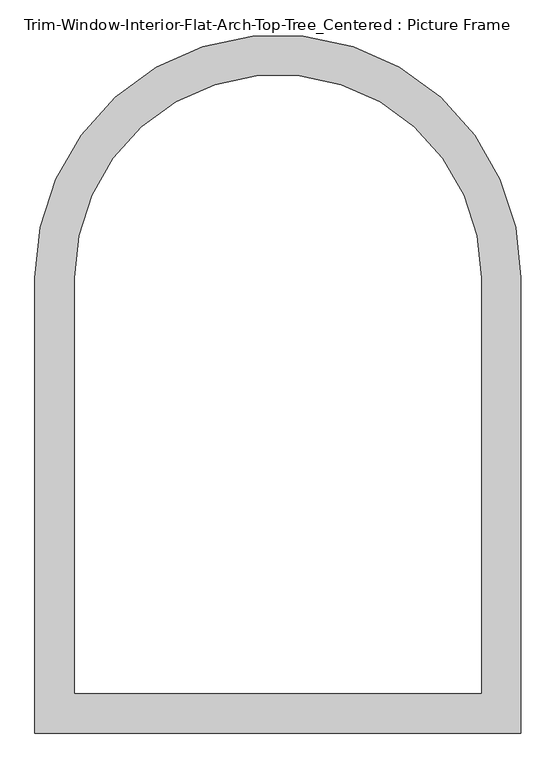
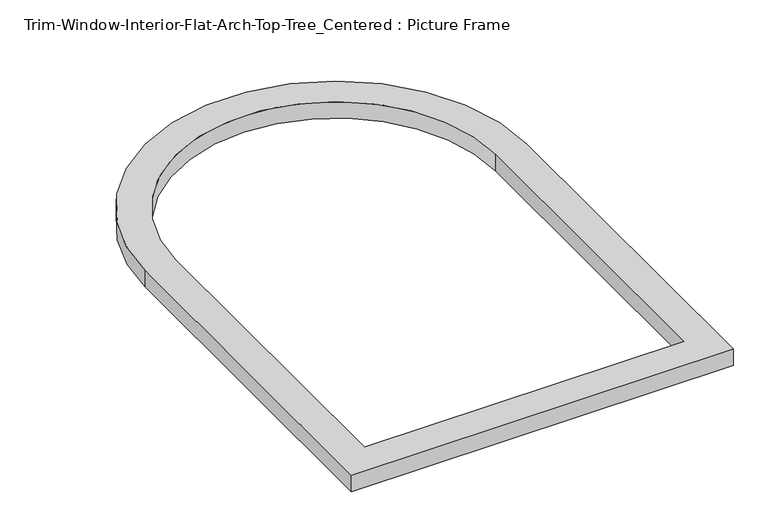
"""IFC4 building model written with IfcOpenShell, lengths in millimetres: proxy geometry, Trim-Window-Interior-Flat-Arch-Top-Tree_Centered : Picture Frame."""

from ifc_helpers import new_model, si_unit, point, frame_2d, origin, origin_with_axes, place, context, project, spatial, polyline, circle_curve, trimmed, segment, composite_curve, outline, extrude, source, transform, mapped, element, save


def trim_window_interior_flat_arch_top_tree_centered_picture_1d59b3d4(model_context):
    return source(origin(), model_context, "Body", "SweptSolid", [
        extrude(outline(composite_curve([segment(trimmed(circle_curve(frame_2d((0.0, -304.8)), 349.25), [point((-349.25, -304.8))], [point((349.25, -304.8))], False, "CARTESIAN"), True, "CONTINUOUS"), segment(polyline([(349.25, -304.8), (349.25, -958.85), (-349.25, -958.85), (-349.25, -304.8)]), True, "CONTINUOUS")], self_intersect=False), holes=[composite_curve([segment(polyline([(-292.1, -304.8), (-292.1, -901.7), (292.1, -901.7), (292.1, -304.8)]), True, "CONTINUOUS"), segment(trimmed(circle_curve(frame_2d((0.0, -304.8)), 292.1), [point((292.1, -304.8))], [point((-292.1, -304.8))], True, "CARTESIAN"), True, "CONTINUOUS")], self_intersect=False)]), origin_with_axes(), (0.0, 0.0, 1.0), 31.75),
    ])


if __name__ == "__main__":
    model = new_model("IFC4")
    model_context = context("Model", 3, world=origin())
    ifc_project = project(units=[si_unit("LENGTHUNIT", "METRE", prefix="MILLI")], contexts=[model_context])
    site = spatial("IfcSite", under=ifc_project)
    building = spatial("IfcBuilding", under=site)
    placement = place(None, origin())
    trim_window_interior_flat_arch_top_tree_centered_picture_shape = trim_window_interior_flat_arch_top_tree_centered_picture_1d59b3d4(model_context)
    element("IfcBuildingElementProxy", 1, Name="Trim-Window-Interior-Flat-Arch-Top-Tree_Centered : Picture Frame", ObjectType="Trim-Window-Interior-Flat-Arch-Top-Tree_Centered : Picture Frame", at=placement, inside=building, context=model_context, shape_type="MappedRepresentation", body=[
        mapped(trim_window_interior_flat_arch_top_tree_centered_picture_shape, transform((0.0, 0.0, 0.0), x_axis=(1.0, 0.0, 0.0), y_axis=(0.0, 1.0, 0.0), z_axis=(0.0, 0.0, 1.0))),
    ])
    save(model, "model.ifc")

# Revit data of these elements
# Type "Trim-Window-Interior-Flat-Arch-Top-Tree_Centered : Picture Frame"
#   Trim Thickness_Picture Frame = 0' - 1 1/4"
#   Trim Width = 0' - 2 1/4"
#   Trim Thickness_with Sill = 0' - 0 3/4"
#   Sill Thickness = 0' - 1 1/4"
#   Opening Width [instance default] = 2' - 0"
#   Opening Height [instance default] = 3' - 0"
#   Default Elevation = 4' - 0"
#   Sill = no
#   Picture Frame = yes
#   Trim Material [instance default] = none
# Element 1 (IfcBuildingElementProxy, "Trim-Window-Interior-Flat-Arch-Top-Tree_Centered : Picture Frame")
#   Trim Material = Wood - Stained
#   Materials on its faces: "Wood - Stained"
# Materials
#   "Wood - Stained": class "Wood", colour RGB 224 178 126, transparency 0, Cost = 0
